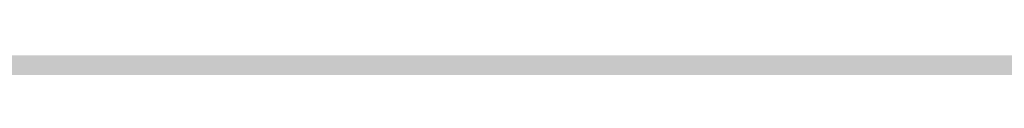
# Model space of a CAD drawing. Units: millimetres. Extents: x 0 to 2267, y 0 to 1823.
# Tile 180 of 256: x 1838.83 to 1841.442, y 1127.384 to 1127.404. Entities that reach past the tile are written whole.
import ezdxf

# ---------------------------------------------------------------- set-up
doc = ezdxf.new("R2010")
doc.units = ezdxf.units.MM
doc.header["$MEASUREMENT"] = 0
doc.layers.add('M-DIMS', color=2, linetype='Continuous', lineweight=25)
doc.layers.add('M-HATC', color=252, linetype='Continuous', lineweight=18)
doc.styles.get("Standard").update_dxf_attribs({"font": 'arial.ttf'})
doc.dimstyles.get("Standard").update_dxf_attribs({"dimtxt": 7, "dimasz": 4, "dimexe": 0.18, "dimexo": 0.0625, "dimgap": 0.09, "dimtad": 0, "dimdec": 0, "dimzin": 0, "dimdsep": 46, "dimtxsty": 'Standard', "dimcen": 0.09, "dimadec": 0, "dimazin": 0, "dimtfac": 1, "dimtdec": 0, "dimtofl": 0, "dimtmove": 0, "dimatfit": 3, "dimfxl": 1, "dimtolj": 1, "dimtzin": 0, "dimarcsym": 0})

# ---------------------------------------------------------------- blocks, each defined once
blk = doc.blocks.new('*D1')
at = {"layer": 'Defpoints', "color": 0, "transparency": 16777216}
for p in [(1593.4289, 1127.4171), (1843.4289, 1127.4171), (1843.4289, 955.6278)]:
    blk.add_point(p, dxfattribs=at)
at = {"layer": 'M-DIMS', "color": 0, "lineweight": -2, "transparency": 16777216}
for p, q in [((1593.4289, 1127.3546), (1593.4289, 955.4478)), ((1843.4289, 1127.3546), (1843.4289, 955.4478)), ((1597.4289, 955.6278), (1710.5582, 955.6278)), ((1839.4289, 955.6278), (1726.2996, 955.6278))]:
    blk.add_line(p, q, dxfattribs=at)
at = {"layer": 'M-DIMS', "color": 0, "transparency": 16777216}
for points in [[(1597.4289, 956.2944), (1597.4289, 954.9611), (1593.4289, 955.6278)], [(1839.4289, 956.2944), (1839.4289, 954.9611), (1843.4289, 955.6278)]]:
    blk.add_solid(points, dxfattribs=at)
at = {"layer": 'M-DIMS', "color": 0, "transparency": 16777216, "insert": (1718.4289, 955.6278), "char_height": 7, "attachment_point": 5}
blk.add_mtext('\\A1;250', dxfattribs=at)

msp = doc.modelspace()

# ---------------------------------------------------------------- hatches: boundary and pattern name
at = {"layer": 'M-HATC'}
h = msp.add_hatch(color=256, dxfattribs=at)
h.dxf.hatch_style = 1
h.paths.add_polyline_path([(2055.771, 1603.062), (1381.0868, 1603.062), (1381.0868, 1598.062), (2055.771, 1598.062)])
h.paths.add_polyline_path([(2055.771, 1598.062), (1381.0868, 1598.062), (1381.0868, 1593.062), (2055.771, 1593.062)])
h.paths.add_polyline_path([(2051.3074, 1536.7609), (1385.5504, 1536.7609), (1385.5504, 1526.7609), (1387.5504, 1526.7609), (1388.5366, 1525.0528), (1385.3319, 1521.2335), (1385.3319, 1521.2226), (2050.2542, 1522.7491), (2048.3212, 1525.0528), (2049.3074, 1526.7609), (2051.3074, 1526.7609)])
edge = h.paths.add_edge_path()
edge.add_arc((1847.5345, 1379.1492), 135, 222.603061, 222.890851, ccw=False)
edge.add_line((1748.1663, 1287.7656), (1683.0921, 1287.7656))
edge.add_arc((1583.7239, 1379.1492), 135, 317.109149, 317.396939, ccw=False)
edge.add_arc((1678.9686, 1290.6707), 5, 222.8909, 317.1091, ccw=False)
edge.add_arc((1774.2133, 1379.1492), 135, 222.603061, 222.890851, ccw=False)
edge.add_line((1674.8451, 1287.7656), (1609.7709, 1287.7656))
edge.add_arc((1510.4027, 1379.1492), 135, 317.109149, 317.396939, ccw=False)
edge.add_arc((1605.6474, 1290.6707), 5, 222.8909, 317.1091, ccw=False)
edge.add_arc((1700.8921, 1379.1492), 135, 222.603061, 222.890851, ccw=False)
edge.add_line((1601.5239, 1287.7656), (1536.4497, 1287.7656))
edge.add_arc((1437.0815, 1379.1492), 135, 317.109149, 317.396939, ccw=False)
edge.add_arc((1532.3262, 1290.6707), 5, 222.8909, 317.1091, ccw=False)
edge.add_arc((1627.5709, 1379.1492), 135, 222.603061, 222.890851, ccw=False)
edge.add_line((1528.2027, 1287.7656), (1505.9289, 1287.7656))
edge.add_spline(control_points=[(1505.9289, 1287.7656), (1504.2622, 1287.7656), (1504.2622, 1282.7656), (1505.9289, 1282.7656)], knot_values=[0, 0, 0, 0, 5, 5, 5, 5], degree=3, periodic=0)
edge.add_line((1505.9289, 1282.7656), (1930.9289, 1282.7656))
edge.add_spline(control_points=[(1930.9289, 1282.7656), (1932.5956, 1282.7656), (1932.5956, 1287.7656), (1930.9289, 1287.7656)], knot_values=[0, 0, 0, 0, 5, 5, 5, 5], degree=3, periodic=0)
edge.add_line((1930.9289, 1287.7656), (1903.0557, 1287.7656))
edge.add_arc((1803.6875, 1379.1492), 135, 317.109149, 317.396939, ccw=False)
edge.add_arc((1898.9322, 1290.6707), 5, 222.8909, 317.1091, ccw=False)
edge.add_arc((1994.1769, 1379.1492), 135, 222.603061, 222.890851, ccw=False)
edge.add_line((1894.8087, 1287.7656), (1829.7345, 1287.7656))
edge.add_arc((1730.3663, 1379.1492), 135, 317.109149, 317.396939, ccw=False)
edge.add_arc((1825.611, 1290.6707), 5, 222.8909, 317.1091, ccw=False)
edge.add_arc((1920.8557, 1379.1492), 135, 222.603061, 222.890851, ccw=False)
edge.add_line((1821.4875, 1287.7656), (1756.4133, 1287.7656))
edge.add_arc((1657.0451, 1379.1492), 135, 317.109149, 317.396939, ccw=False)
edge.add_arc((1752.2898, 1290.6707), 5, 222.8909, 317.1091, ccw=False)
edge = h.paths.add_edge_path()
edge.add_spline(control_points=[(1843.4289, 1227.2475), (1845.0956, 1227.2475), (1845.0956, 1232.2475), (1843.4289, 1232.2475)], knot_values=[0, 0, 0, 0, 5, 5, 5, 5], degree=3, periodic=0)
edge.add_line((1843.4289, 1232.2475), (1593.4289, 1232.2475))
edge.add_spline(control_points=[(1593.4289, 1232.2475), (1591.7622, 1232.2475), (1591.7622, 1227.2475), (1593.4289, 1227.2475)], knot_values=[0, 0, 0, 0, 5, 5, 5, 5], degree=3, periodic=0)
edge.add_line((1593.4289, 1227.2475), (1843.4289, 1227.2475))
h.paths.add_polyline_path([(1905.9289, 1127.4171), (1530.9289, 1127.4171, 0.414214), (1520.9289, 1117.4171), (1530.9289, 1117.4171), (1915.9289, 1117.4171, 0.414214)])
edge = h.paths.add_edge_path()
edge.add_arc((1397.0858, 1498.4078), 12.7299, 90.78215, 190.87871, ccw=False)
edge.add_line((1396.912, 1511.1365), (1428.0097, 1511.3488))
edge.add_line((1428.0097, 1511.3488), (1433.0097, 1511.3488))
edge.add_line((1433.0097, 1511.3488), (1434.439, 1511.3488))
edge.add_arc((1419.474, 1498.0804), 20, 41.561, 74.08211)
edge.add_line((1424.9592, 1517.3135), (1399.9351, 1517.2561))
edge.add_spline(control_points=[(1399.9307, 1517.2561), (1399.884, 1517.2131), (1399.8328, 1517.1689), (1399.7774, 1517.1236)], knot_values=[11.567499, 11.567499, 11.567499, 11.567499, 11.814249, 11.814249, 11.814249, 11.814249], degree=3, periodic=0)
edge.add_spline(control_points=[(1399.6328, 1517.0099), (1399.5831, 1516.9721), (1399.5307, 1516.9338), (1399.4759, 1516.8947)], knot_values=[11.167718, 11.167718, 11.167718, 11.167718, 11.365188, 11.365188, 11.365188, 11.365188], degree=3, periodic=0)
edge.add_spline(control_points=[(1399.3398, 1516.8001), (1399.1514, 1516.6719), (1398.9384, 1516.5377), (1398.704, 1516.3994)], knot_values=[10.376405, 10.376405, 10.376405, 10.376405, 11.00994, 11.00994, 11.00994, 11.00994], degree=3, periodic=0)
edge.add_spline(control_points=[(1398.6572, 1516.3719), (1398.5789, 1516.326), (1398.4983, 1516.2797), (1398.4155, 1516.2331)], knot_values=[10.125175, 10.125175, 10.125175, 10.125175, 10.334406, 10.334406, 10.334406, 10.334406], degree=3, periodic=0)
edge.add_spline(control_points=[(1398.2642, 1516.1487), (1398.196, 1516.1111), (1398.1263, 1516.0732), (1398.0555, 1516.0351)], knot_values=[9.832246, 9.832246, 9.832246, 9.832246, 9.999658, 9.999658, 9.999658, 9.999658], degree=3, periodic=0)
edge.add_spline(control_points=[(1397.9987, 1516.0048), (1397.7312, 1515.8621), (1397.446, 1515.7171), (1397.1466, 1515.5714)], knot_values=[9.161808, 9.161808, 9.161808, 9.161808, 9.787769, 9.787769, 9.787769, 9.787769], degree=3, periodic=0)
edge.add_spline(control_points=[(1397.1466, 1515.5714), (1396.8418, 1515.423), (1396.5222, 1515.274), (1396.1914, 1515.1262)], knot_values=[8.524455, 8.524455, 8.524455, 8.524455, 9.161808, 9.161808, 9.161808, 9.161808], degree=3, periodic=0)
edge.add_spline(control_points=[(1396.0777, 1515.0756), (1395.9854, 1515.0348), (1395.8922, 1514.994), (1395.7983, 1514.9534)], knot_values=[8.275193, 8.275193, 8.275193, 8.275193, 8.451726, 8.451726, 8.451726, 8.451726], degree=3, periodic=0)
edge.add_spline(control_points=[(1395.6018, 1514.8691), (1395.4997, 1514.8257), (1395.3968, 1514.7824), (1395.2932, 1514.7394)], knot_values=[7.962917, 7.962917, 7.962917, 7.962917, 8.152764, 8.152764, 8.152764, 8.152764], degree=3, periodic=0)
edge.add_spline(control_points=[(1395.2116, 1514.7057), (1394.8278, 1514.5475), (1394.4345, 1514.3929), (1394.0364, 1514.2442)], knot_values=[7.21254, 7.21254, 7.21254, 7.21254, 7.913148, 7.913148, 7.913148, 7.913148], degree=3, periodic=0)
edge.add_spline(control_points=[(1394.0364, 1514.2442), (1393.7076, 1514.1214), (1393.3754, 1514.0027), (1393.0427, 1513.8895)], knot_values=[6.633733, 6.633733, 6.633733, 6.633733, 7.21254, 7.21254, 7.21254, 7.21254], degree=3, periodic=0)
edge.add_spline(control_points=[(1392.8214, 1513.815), (1392.7198, 1513.7812), (1392.6181, 1513.7479), (1392.5166, 1513.7152)], knot_values=[6.328796, 6.328796, 6.328796, 6.328796, 6.505493, 6.505493, 6.505493, 6.505493], degree=3, periodic=0)
edge.add_spline(control_points=[(1392.5166, 1513.7152), (1392.3187, 1513.6515), (1392.1212, 1513.59), (1391.9244, 1513.531)], knot_values=[5.984605, 5.984605, 5.984605, 5.984605, 6.328796, 6.328796, 6.328796, 6.328796], degree=3, periodic=0)
edge.add_spline(control_points=[(1391.7915, 1513.4915), (1391.3122, 1513.3501), (1390.8384, 1513.2239), (1390.3784, 1513.1171)], knot_values=[5.066697, 5.066697, 5.066697, 5.066697, 5.907055, 5.907055, 5.907055, 5.907055], degree=3, periodic=0)
edge.add_spline(control_points=[(1390.3784, 1513.1171), (1390.1797, 1513.071), (1389.9836, 1513.0284), (1389.7907, 1512.9899)], knot_values=[4.70367, 4.70367, 4.70367, 4.70367, 5.066695, 5.066695, 5.066695, 5.066695], degree=3, periodic=0)
edge.add_spline(control_points=[(1389.422, 1512.9204), (1389.2459, 1512.8892), (1389.0729, 1512.8617), (1388.9036, 1512.8381)], knot_values=[4.130571, 4.130571, 4.130571, 4.130571, 4.469816, 4.469816, 4.469816, 4.469816], degree=3, periodic=0)
edge.add_spline(control_points=[(1388.9036, 1512.8381), (1388.591, 1512.7946), (1388.2911, 1512.7644), (1388.0071, 1512.7494)], knot_values=[3.504031, 3.504031, 3.504031, 3.504031, 4.130571, 4.130571, 4.130571, 4.130571], degree=3, periodic=0)
edge.add_spline(control_points=[(1387.9356, 1512.7459), (1387.8538, 1512.7423), (1387.7733, 1512.74), (1387.6944, 1512.739)], knot_values=[3.268866, 3.268866, 3.268866, 3.268866, 3.451164, 3.451164, 3.451164, 3.451164], degree=3, periodic=0)
edge.add_spline(control_points=[(1387.3351, 1512.7443), (1387.2076, 1512.7499), (1387.0847, 1512.7597), (1386.967, 1512.7739)], knot_values=[2.670686, 2.670686, 2.670686, 2.670686, 2.984, 2.984, 2.984, 2.984], degree=3, periodic=0)
edge.add_spline(control_points=[(1386.8327, 1512.7922), (1386.8209, 1512.7941), (1386.8092, 1512.7959), (1386.7975, 1512.7979)], knot_values=[2.516981, 2.516981, 2.516981, 2.516981, 2.549528, 2.549528, 2.549528, 2.549528], degree=3, periodic=0)
edge.add_spline(control_points=[(1386.4526, 1512.8735), (1386.4257, 1512.881), (1386.3993, 1512.889), (1386.3733, 1512.8972)], knot_values=[2.095869, 2.095869, 2.095869, 2.095869, 2.17941, 2.17941, 2.17941, 2.17941], degree=3, periodic=0)
edge.add_spline(control_points=[(1386.0691, 1513.0189), (1386.0634, 1513.0217), (1386.0577, 1513.0246), (1386.052, 1513.0275)], knot_values=[1.72453, 1.72453, 1.72453, 1.72453, 1.745933, 1.745933, 1.745933, 1.745933], degree=3, periodic=0)
edge.add_arc((1399.474, 1498.0804), 20, 131.82432, 180)
edge.add_arc((1630.3336, 1505.5484), 250.9708, 181.705176, 236.427975)
edge.add_arc((1605.3399, 1483.3044), 218.7822, 238.660829, 243.34961)
edge.add_arc((1647.0911, 1510.3592), 262.8986, 183.129836, 237.853442, ccw=False)
h.paths.add_polyline_path([(1406.5369, 1391.9644, 0.149382), (1491.5506, 1296.4418, -0.129517)], flags=17)
edge = h.paths.add_edge_path()
edge.add_arc((2037.3838, 1498.0804), 20, 0, 48.26587)
edge.add_spline(control_points=[(2050.6973, 1513.0052), (2050.6512, 1512.9847), (2050.6034, 1512.9655), (2050.5539, 1512.9477)], knot_values=[1.835652, 1.835652, 1.835652, 1.835652, 2.000781, 2.000781, 2.000781, 2.000781], degree=3, periodic=0)
edge.add_spline(control_points=[(2050.4616, 1512.9166), (2050.479, 1512.9221), (2050.4963, 1512.9277), (2050.5133, 1512.9335)], knot_values=[2.045477, 2.045477, 2.045477, 2.045477, 2.101389, 2.101389, 2.101389, 2.101389], degree=3, periodic=0)
edge.add_spline(control_points=[(2050.129, 1512.8342), (2050.1984, 1512.8473), (2050.2657, 1512.8623), (2050.3308, 1512.8792)], knot_values=[2.237629, 2.237629, 2.237629, 2.237629, 2.435841, 2.435841, 2.435841, 2.435841], degree=3, periodic=0)
edge.add_spline(control_points=[(2050.0946, 1512.8278), (2050.1061, 1512.8299), (2050.1176, 1512.832), (2050.129, 1512.8342)], knot_values=[2.435841, 2.435841, 2.435841, 2.435841, 2.468321, 2.468321, 2.468321, 2.468321], degree=3, periodic=0)
edge.add_spline(control_points=[(2049.7843, 1512.7851), (2049.8552, 1512.7922), (2049.9243, 1512.8008), (2049.9917, 1512.8109)], knot_values=[2.563852, 2.563852, 2.563852, 2.563852, 2.748541, 2.748541, 2.748541, 2.748541], degree=3, periodic=0)
edge.add_spline(control_points=[(2049.4052, 1512.7617), (2049.5364, 1512.7653), (2049.6629, 1512.773), (2049.7843, 1512.7851)], knot_values=[2.748541, 2.748541, 2.748541, 2.748541, 3.064882, 3.064882, 3.064882, 3.064882], degree=3, periodic=0)
edge.add_spline(control_points=[(2049.1698, 1512.7597), (2049.2336, 1512.7591), (2049.2965, 1512.7594), (2049.3584, 1512.7606)], knot_values=[3.102309, 3.102309, 3.102309, 3.102309, 3.2503, 3.2503, 3.2503, 3.2503], degree=3, periodic=0)
edge.add_spline(control_points=[(2048.8573, 1512.7691), (2048.9638, 1512.7638), (2049.068, 1512.7606), (2049.1698, 1512.7597)], knot_values=[3.2503, 3.2503, 3.2503, 3.2503, 3.486069, 3.486069, 3.486069, 3.486069], degree=3, periodic=0)
edge.add_spline(control_points=[(2048.6924, 1512.7789), (2048.3729, 1512.8009), (2048.0345, 1512.8411), (2047.6817, 1512.897)], knot_values=[3.606429, 3.606429, 3.606429, 3.606429, 4.2989, 4.2989, 4.2989, 4.2989], degree=3, periodic=0)
edge.add_spline(control_points=[(2047.6817, 1512.897), (2047.5458, 1512.9185), (2047.4077, 1512.9424), (2047.2678, 1512.9685)], knot_values=[4.2989, 4.2989, 4.2989, 4.2989, 4.565769, 4.565769, 4.565769, 4.565769], degree=3, periodic=0)
edge.add_spline(control_points=[(2047.2678, 1512.9685), (2047.1449, 1512.9914), (2047.0207, 1513.016), (2046.8951, 1513.0422)], knot_values=[4.565769, 4.565769, 4.565769, 4.565769, 4.799971, 4.799971, 4.799971, 4.799971], degree=3, periodic=0)
edge.add_spline(control_points=[(2046.8951, 1513.0422), (2046.5286, 1513.1188), (2046.1513, 1513.209), (2045.7676, 1513.3107)], knot_values=[4.799971, 4.799971, 4.799971, 4.799971, 5.483718, 5.483718, 5.483718, 5.483718], degree=3, periodic=0)
edge.add_spline(control_points=[(2045.7676, 1513.3107), (2045.3724, 1513.4154), (2044.9704, 1513.5322), (2044.5662, 1513.6588)], knot_values=[5.483718, 5.483718, 5.483718, 5.483718, 6.187866, 6.187866, 6.187866, 6.187866], degree=3, periodic=0)
edge.add_spline(control_points=[(2044.5662, 1513.6588), (2044.4149, 1513.7061), (2044.2633, 1513.7549), (2044.1116, 1513.8048)], knot_values=[6.187866, 6.187866, 6.187866, 6.187866, 6.451551, 6.451551, 6.451551, 6.451551], degree=3, periodic=0)
edge.add_spline(control_points=[(2044.1116, 1513.8048), (2043.9967, 1513.8427), (2043.8817, 1513.8813), (2043.7668, 1513.9205)], knot_values=[6.451551, 6.451551, 6.451551, 6.451551, 6.651434, 6.651434, 6.651434, 6.651434], degree=3, periodic=0)
edge.add_spline(control_points=[(2043.7668, 1513.9205), (2043.3716, 1514.0554), (2042.9774, 1514.1979), (2042.5886, 1514.3458)], knot_values=[6.651434, 6.651434, 6.651434, 6.651434, 7.338879, 7.338879, 7.338879, 7.338879], degree=3, periodic=0)
edge.add_spline(control_points=[(2042.5886, 1514.3458), (2042.1643, 1514.5071), (2041.7465, 1514.6749), (2041.3409, 1514.846)], knot_values=[7.338879, 7.338879, 7.338879, 7.338879, 8.089209, 8.089209, 8.089209, 8.089209], degree=3, periodic=0)
edge.add_spline(control_points=[(2041.3409, 1514.846), (2041.1028, 1514.9465), (2040.869, 1515.0481), (2040.6405, 1515.1502)], knot_values=[8.089209, 8.089209, 8.089209, 8.089209, 8.529587, 8.529587, 8.529587, 8.529587], degree=3, periodic=0)
edge.add_spline(control_points=[(2040.51, 1515.2089), (2040.0824, 1515.4022), (2039.6747, 1515.5971), (2039.295, 1515.7894)], knot_values=[8.613818, 8.613818, 8.613818, 8.613818, 9.44571, 9.44571, 9.44571, 9.44571], degree=3, periodic=0)
edge.add_spline(control_points=[(2039.295, 1515.7894), (2039.0618, 1515.9075), (2038.8391, 1516.0246), (2038.6288, 1516.1398)], knot_values=[9.44571, 9.44571, 9.44571, 9.44571, 9.956404, 9.956404, 9.956404, 9.956404], degree=3, periodic=0)
edge.add_spline(control_points=[(2038.6288, 1516.1398), (2038.5187, 1516.2001), (2038.4121, 1516.2598), (2038.309, 1516.3189)], knot_values=[9.956404, 9.956404, 9.956404, 9.956404, 10.223542, 10.223542, 10.223542, 10.223542], degree=3, periodic=0)
edge.add_spline(control_points=[(2038.309, 1516.3189), (2038.2138, 1516.3735), (2038.1216, 1516.4276), (2038.0328, 1516.481)], knot_values=[10.223542, 10.223542, 10.223542, 10.223542, 10.47051, 10.47051, 10.47051, 10.47051], degree=3, periodic=0)
edge.add_spline(control_points=[(2038.0328, 1516.481), (2037.7855, 1516.6296), (2037.5639, 1516.773), (2037.3722, 1516.909)], knot_values=[10.47051, 10.47051, 10.47051, 10.47051, 11.15767, 11.15767, 11.15767, 11.15767], degree=3, periodic=0)
edge.add_spline(control_points=[(2037.3722, 1516.909), (2037.2789, 1516.9752), (2037.1927, 1517.0396), (2037.1142, 1517.102)], knot_values=[11.15767, 11.15767, 11.15767, 11.15767, 11.49227, 11.49227, 11.49227, 11.49227], degree=3, periodic=0)
edge.add_spline(control_points=[(2036.8564, 1517.3259), (2036.9148, 1517.2692), (2036.9814, 1517.2103), (2037.0557, 1517.1492)], knot_values=[11.577341, 11.577341, 11.577341, 11.577341, 11.91035, 11.91035, 11.91035, 11.91035], degree=3, periodic=0)
edge.add_spline(control_points=[(2036.8074, 1517.3748), (2036.823, 1517.3587), (2036.8393, 1517.3424), (2036.8564, 1517.3259)], knot_values=[11.91035, 11.91035, 11.91035, 11.91035, 12.007402, 12.007402, 12.007402, 12.007402], degree=3, periodic=0)
edge.add_spline(control_points=[(2036.7017, 1517.494), (2036.7104, 1517.483), (2036.7196, 1517.4719), (2036.7291, 1517.4606)], knot_values=[12.184155, 12.184155, 12.184155, 12.184155, 12.255409, 12.255409, 12.255409, 12.255409], degree=3, periodic=0)
edge.add_spline(control_points=[(2036.6159, 1517.6205), (2036.62, 1517.613), (2036.6243, 1517.6055), (2036.6289, 1517.5979)], knot_values=[12.487913, 12.487913, 12.487913, 12.487913, 12.541035, 12.541035, 12.541035, 12.541035], degree=3, periodic=0)
edge.add_spline(control_points=[(2036.5635, 1517.786), (2036.5637, 1517.7794), (2036.5642, 1517.7726), (2036.565, 1517.7658)], knot_values=[12.911761, 12.911761, 12.911761, 12.911761, 12.968286, 12.968286, 12.968286, 12.968286], degree=3, periodic=0)
edge.add_spline(control_points=[(2036.6166, 1517.9304), (2036.6125, 1517.9259), (2036.6086, 1517.9212), (2036.6049, 1517.9165)], knot_values=[13.382527, 13.382527, 13.382527, 13.382527, 13.433791, 13.433791, 13.433791, 13.433791], degree=3, periodic=0)
edge.add_spline(control_points=[(2036.749, 1518.017), (2036.7361, 1518.0116), (2036.7239, 1518.006), (2036.7124, 1518.0002)], knot_values=[13.726299, 13.726299, 13.726299, 13.726299, 13.809928, 13.809928, 13.809928, 13.809928], degree=3, periodic=0)
edge.add_spline(control_points=[(2036.8604, 1518.0528), (2036.8386, 1518.0474), (2036.8181, 1518.0416), (2036.7988, 1518.0353)], knot_values=[13.910887, 13.910887, 13.910887, 13.910887, 14.02153, 14.02153, 14.02153, 14.02153], degree=3, periodic=0)
edge.add_line((2036.9639, 1518.0804), (2032.3838, 1518.0804))
edge.add_line((2032.3838, 1518.0804), (2027.3838, 1518.0804))
edge.add_line((2027.3838, 1518.0804), (2022.3838, 1518.0804))
edge.add_line((2022.3838, 1518.0804), (2017.3838, 1518.0804))
edge.add_arc((2017.3838, 1498.0804), 20, 90, 138.439)
edge.add_line((2002.4188, 1511.3488), (2003.8481, 1511.3488))
edge.add_line((2003.8481, 1511.3488), (2008.8481, 1511.3488))
edge.add_line((2008.8481, 1511.3488), (2039.772, 1511.1377))
edge.add_arc((2039.772, 1498.4078), 12.7299, -10.87871, 90, ccw=False)
edge.add_arc((1789.7668, 1510.3592), 262.8986, 302.146558, 356.870164, ccw=False)
edge.add_arc((1831.5179, 1483.3044), 218.7822, 296.65039, 301.339171)
edge.add_arc((1806.5242, 1505.5484), 250.9708, 303.572025, 358.294824)
h.paths.add_polyline_path([(2030.321, 1391.9644, -0.129517), (1945.3072, 1296.4418, 0.149382)], flags=17)
edge = h.paths.add_edge_path()
edge.add_spline(control_points=[(2037.2464, 1518.0821), (2037.2898, 1518.081), (2037.3355, 1518.0804), (2037.3838, 1518.0804)], knot_values=[0.000012, 0.000012, 0.000012, 0.000012, 0.144754, 0.144754, 0.144754, 0.144754], degree=3, periodic=0)
edge.add_line((2037.3357, 1518.0804), (2037.0096, 1518.0804))
edge.add_spline(control_points=[(2037.0096, 1518.0804), (2036.9822, 1518.0768), (2036.956, 1518.0727), (2036.9312, 1518.0681)], knot_values=[14.13465, 14.13465, 14.13465, 14.13465, 14.247197, 14.247197, 14.247197, 14.247197], degree=3, periodic=0)
edge.add_spline(control_points=[(2036.9312, 1518.0681), (2036.9276, 1518.0674), (2036.9241, 1518.0667), (2036.9205, 1518.0661)], knot_values=[14.118315, 14.118315, 14.118315, 14.118315, 14.13465, 14.13465, 14.13465, 14.13465], degree=3, periodic=0)
edge.add_spline(control_points=[(2036.9205, 1518.0661), (2036.9118, 1518.0644), (2036.9032, 1518.0626), (2036.8948, 1518.0608)], knot_values=[14.078086, 14.078086, 14.078086, 14.078086, 14.118315, 14.118315, 14.118315, 14.118315], degree=3, periodic=0)
edge.add_spline(control_points=[(2036.8948, 1518.0608), (2036.883, 1518.0583), (2036.8716, 1518.0556), (2036.8604, 1518.0528)], knot_values=[14.02153, 14.02153, 14.02153, 14.02153, 14.078086, 14.078086, 14.078086, 14.078086], degree=3, periodic=0)
edge.add_spline(control_points=[(2036.8604, 1518.0528), (2036.8386, 1518.0474), (2036.8181, 1518.0416), (2036.7988, 1518.0353)], knot_values=[13.910887, 13.910887, 13.910887, 13.910887, 14.02153, 14.02153, 14.02153, 14.02153], degree=3, periodic=0)
edge.add_spline(control_points=[(2036.7988, 1518.0353), (2036.7981, 1518.035), (2036.7974, 1518.0348), (2036.7967, 1518.0346)], knot_values=[13.906906, 13.906906, 13.906906, 13.906906, 13.910887, 13.910887, 13.910887, 13.910887], degree=3, periodic=0)
edge.add_spline(control_points=[(2036.7967, 1518.0346), (2036.7882, 1518.0318), (2036.7799, 1518.0289), (2036.7719, 1518.0259)], knot_values=[13.857826, 13.857826, 13.857826, 13.857826, 13.906906, 13.906906, 13.906906, 13.906906], degree=3, periodic=0)
edge.add_spline(control_points=[(2036.7719, 1518.0259), (2036.764, 1518.023), (2036.7564, 1518.02), (2036.749, 1518.017)], knot_values=[13.809928, 13.809928, 13.809928, 13.809928, 13.857826, 13.857826, 13.857826, 13.857826], degree=3, periodic=0)
edge.add_spline(control_points=[(2036.749, 1518.017), (2036.7361, 1518.0116), (2036.7239, 1518.006), (2036.7124, 1518.0002)], knot_values=[13.726299, 13.726299, 13.726299, 13.726299, 13.809928, 13.809928, 13.809928, 13.809928], degree=3, periodic=0)
edge.add_spline(control_points=[(2036.7124, 1518.0002), (2036.7121, 1518), (2036.7118, 1517.9999), (2036.7115, 1517.9997)], knot_values=[13.723993, 13.723993, 13.723993, 13.723993, 13.726299, 13.726299, 13.726299, 13.726299], degree=3, periodic=0)
edge.add_spline(control_points=[(2036.7115, 1517.9997), (2036.7063, 1517.9971), (2036.7013, 1517.9944), (2036.6965, 1517.9917)], knot_values=[13.686536, 13.686536, 13.686536, 13.686536, 13.723993, 13.723993, 13.723993, 13.723993], degree=3, periodic=0)
edge.add_spline(control_points=[(2036.6965, 1517.9917), (2036.6919, 1517.9891), (2036.6874, 1517.9865), (2036.6831, 1517.9839)], knot_values=[13.651251, 13.651251, 13.651251, 13.651251, 13.686536, 13.686536, 13.686536, 13.686536], degree=3, periodic=0)
edge.add_spline(control_points=[(2036.6831, 1517.9839), (2036.6764, 1517.9798), (2036.67, 1517.9757), (2036.6639, 1517.9714)], knot_values=[13.596804, 13.596804, 13.596804, 13.596804, 13.651251, 13.651251, 13.651251, 13.651251], degree=3, periodic=0)
edge.add_spline(control_points=[(2036.6639, 1517.9714), (2036.6636, 1517.9712), (2036.6633, 1517.9709), (2036.6629, 1517.9707)], knot_values=[13.593956, 13.593956, 13.593956, 13.593956, 13.596804, 13.596804, 13.596804, 13.596804], degree=3, periodic=0)
edge.add_spline(control_points=[(2036.6629, 1517.9707), (2036.6603, 1517.9689), (2036.6577, 1517.967), (2036.6552, 1517.9651)], knot_values=[13.570322, 13.570322, 13.570322, 13.570322, 13.593956, 13.593956, 13.593956, 13.593956], degree=3, periodic=0)
edge.add_spline(control_points=[(2036.6552, 1517.9651), (2036.6525, 1517.9631), (2036.6499, 1517.9611), (2036.6474, 1517.9591)], knot_values=[13.545477, 13.545477, 13.545477, 13.545477, 13.570322, 13.570322, 13.570322, 13.570322], degree=3, periodic=0)
edge.add_spline(control_points=[(2036.6474, 1517.9591), (2036.6472, 1517.9589), (2036.6471, 1517.9588), (2036.6469, 1517.9587)], knot_values=[13.543931, 13.543931, 13.543931, 13.543931, 13.545477, 13.545477, 13.545477, 13.545477], degree=3, periodic=0)
edge.add_spline(control_points=[(2036.6469, 1517.9587), (2036.6412, 1517.9541), (2036.6358, 1517.9494), (2036.6307, 1517.9447)], knot_values=[13.488237, 13.488237, 13.488237, 13.488237, 13.543931, 13.543931, 13.543931, 13.543931], degree=3, periodic=0)
edge.add_spline(control_points=[(2036.6307, 1517.9447), (2036.6282, 1517.9423), (2036.6257, 1517.9399), (2036.6233, 1517.9374)], knot_values=[13.460307, 13.460307, 13.460307, 13.460307, 13.488237, 13.488237, 13.488237, 13.488237], degree=3, periodic=0)
edge.add_spline(control_points=[(2036.6233, 1517.9374), (2036.6215, 1517.9356), (2036.6198, 1517.9338), (2036.6181, 1517.932)], knot_values=[13.439712, 13.439712, 13.439712, 13.439712, 13.460307, 13.460307, 13.460307, 13.460307], degree=3, periodic=0)
edge.add_spline(control_points=[(2036.6181, 1517.932), (2036.6176, 1517.9315), (2036.6171, 1517.9309), (2036.6166, 1517.9304)], knot_values=[13.433791, 13.433791, 13.433791, 13.433791, 13.439712, 13.439712, 13.439712, 13.439712], degree=3, periodic=0)
edge.add_spline(control_points=[(2036.6166, 1517.9304), (2036.6125, 1517.9259), (2036.6086, 1517.9212), (2036.6049, 1517.9165)], knot_values=[13.382527, 13.382527, 13.382527, 13.382527, 13.433791, 13.433791, 13.433791, 13.433791], degree=3, periodic=0)
edge.add_spline(control_points=[(2036.6049, 1517.9165), (2036.6026, 1517.9135), (2036.6004, 1517.9104), (2036.5982, 1517.9074)], knot_values=[13.350017, 13.350017, 13.350017, 13.350017, 13.382527, 13.382527, 13.382527, 13.382527], degree=3, periodic=0)
edge.add_spline(control_points=[(2036.5982, 1517.9074), (2036.5972, 1517.9059), (2036.5962, 1517.9043), (2036.5952, 1517.9028)], knot_values=[13.333922, 13.333922, 13.333922, 13.333922, 13.350017, 13.350017, 13.350017, 13.350017], degree=3, periodic=0)
edge.add_spline(control_points=[(2036.5952, 1517.9028), (2036.5945, 1517.9018), (2036.5939, 1517.9009), (2036.5933, 1517.8999)], knot_values=[13.323828, 13.323828, 13.323828, 13.323828, 13.333922, 13.333922, 13.333922, 13.333922], degree=3, periodic=0)
edge.add_spline(control_points=[(2036.5933, 1517.8999), (2036.5905, 1517.8955), (2036.5879, 1517.8909), (2036.5855, 1517.8864)], knot_values=[13.277545, 13.277545, 13.277545, 13.277545, 13.323828, 13.323828, 13.323828, 13.323828], degree=3, periodic=0)
edge.add_spline(control_points=[(2036.5855, 1517.8864), (2036.5836, 1517.8827), (2036.5817, 1517.8789), (2036.5801, 1517.8751)], knot_values=[13.240119, 13.240119, 13.240119, 13.240119, 13.277545, 13.277545, 13.277545, 13.277545], degree=3, periodic=0)
edge.add_spline(control_points=[(2036.5801, 1517.8751), (2036.5795, 1517.8739), (2036.579, 1517.8727), (2036.5785, 1517.8715)], knot_values=[13.228211, 13.228211, 13.228211, 13.228211, 13.240119, 13.240119, 13.240119, 13.240119], degree=3, periodic=0)
edge.add_spline(control_points=[(2036.5785, 1517.8715), (2036.578, 1517.8702), (2036.5774, 1517.869), (2036.5769, 1517.8677)], knot_values=[13.215717, 13.215717, 13.215717, 13.215717, 13.228211, 13.228211, 13.228211, 13.228211], degree=3, periodic=0)
edge.add_spline(control_points=[(2036.5769, 1517.8677), (2036.5755, 1517.864), (2036.5741, 1517.8603), (2036.5729, 1517.8565)], knot_values=[13.179847, 13.179847, 13.179847, 13.179847, 13.215717, 13.215717, 13.215717, 13.215717], degree=3, periodic=0)
edge.add_spline(control_points=[(2036.5729, 1517.8565), (2036.5713, 1517.8515), (2036.5699, 1517.8464), (2036.5687, 1517.8413)], knot_values=[13.132017, 13.132017, 13.132017, 13.132017, 13.179847, 13.179847, 13.179847, 13.179847], degree=3, periodic=0)
edge.add_spline(control_points=[(2036.5687, 1517.8413), (2036.5684, 1517.8402), (2036.5682, 1517.8392), (2036.568, 1517.8382)], knot_values=[13.122482, 13.122482, 13.122482, 13.122482, 13.132017, 13.132017, 13.132017, 13.132017], degree=3, periodic=0)
edge.add_spline(control_points=[(2036.568, 1517.8382), (2036.5676, 1517.8363), (2036.5672, 1517.8345), (2036.5669, 1517.8327)], knot_values=[13.105592, 13.105592, 13.105592, 13.105592, 13.122482, 13.122482, 13.122482, 13.122482], degree=3, periodic=0)
edge.add_spline(control_points=[(2036.5669, 1517.8327), (2036.5662, 1517.8292), (2036.5657, 1517.8257), (2036.5652, 1517.8222)], knot_values=[13.074063, 13.074063, 13.074063, 13.074063, 13.105592, 13.105592, 13.105592, 13.105592], degree=3, periodic=0)
edge.add_spline(control_points=[(2036.5652, 1517.8222), (2036.5652, 1517.8222), (2036.5652, 1517.8222), (2036.5652, 1517.8222)], knot_values=[13.074043, 13.074043, 13.074043, 13.074043, 13.074063, 13.074063, 13.074063, 13.074063], degree=3, periodic=0)
edge.add_spline(control_points=[(2036.5652, 1517.8222), (2036.5644, 1517.8164), (2036.5639, 1517.8106), (2036.5636, 1517.8046)], knot_values=[13.021884, 13.021884, 13.021884, 13.021884, 13.074043, 13.074043, 13.074043, 13.074043], degree=3, periodic=0)
edge.add_spline(control_points=[(2036.5636, 1517.8046), (2036.5636, 1517.804), (2036.5636, 1517.8034), (2036.5635, 1517.8028)], knot_values=[13.01674, 13.01674, 13.01674, 13.01674, 13.021884, 13.021884, 13.021884, 13.021884], degree=3, periodic=0)
edge.add_spline(control_points=[(2036.5635, 1517.8028), (2036.5634, 1517.8005), (2036.5634, 1517.7982), (2036.5634, 1517.7958)], knot_values=[12.996438, 12.996438, 12.996438, 12.996438, 13.01674, 13.01674, 13.01674, 13.01674], degree=3, periodic=0)
edge.add_spline(control_points=[(2036.5634, 1517.7958), (2036.5633, 1517.7926), (2036.5634, 1517.7893), (2036.5635, 1517.786)], knot_values=[12.968286, 12.968286, 12.968286, 12.968286, 12.996438, 12.996438, 12.996438, 12.996438], degree=3, periodic=0)
edge.add_spline(control_points=[(2036.5635, 1517.786), (2036.5637, 1517.7794), (2036.5642, 1517.7726), (2036.565, 1517.7658)], knot_values=[12.911761, 12.911761, 12.911761, 12.911761, 12.968286, 12.968286, 12.968286, 12.968286], degree=3, periodic=0)
edge.add_spline(control_points=[(2036.565, 1517.7658), (2036.565, 1517.7657), (2036.565, 1517.7656), (2036.565, 1517.7656)], knot_values=[12.911017, 12.911017, 12.911017, 12.911017, 12.911761, 12.911761, 12.911761, 12.911761], degree=3, periodic=0)
edge.add_spline(control_points=[(2036.565, 1517.7656), (2036.5654, 1517.7625), (2036.5658, 1517.7593), (2036.5663, 1517.7562)], knot_values=[12.88528, 12.88528, 12.88528, 12.88528, 12.911017, 12.911017, 12.911017, 12.911017], degree=3, periodic=0)
edge.add_spline(control_points=[(2036.5663, 1517.7562), (2036.5667, 1517.7534), (2036.5672, 1517.7506), (2036.5677, 1517.7478)], knot_values=[12.862519, 12.862519, 12.862519, 12.862519, 12.88528, 12.88528, 12.88528, 12.88528], degree=3, periodic=0)
edge.add_spline(control_points=[(2036.5677, 1517.7478), (2036.5678, 1517.7474), (2036.5679, 1517.7469), (2036.568, 1517.7465)], knot_values=[12.858885, 12.858885, 12.858885, 12.858885, 12.862519, 12.862519, 12.862519, 12.862519], degree=3, periodic=0)
edge.add_spline(control_points=[(2036.568, 1517.7465), (2036.5692, 1517.7399), (2036.5707, 1517.7332), (2036.5724, 1517.7264)], knot_values=[12.8053, 12.8053, 12.8053, 12.8053, 12.858885, 12.858885, 12.858885, 12.858885], degree=3, periodic=0)
edge.add_spline(control_points=[(2036.5724, 1517.7264), (2036.5734, 1517.7226), (2036.5745, 1517.7187), (2036.5756, 1517.7149)], knot_values=[12.775176, 12.775176, 12.775176, 12.775176, 12.8053, 12.8053, 12.8053, 12.8053], degree=3, periodic=0)
edge.add_spline(control_points=[(2036.5756, 1517.7149), (2036.5763, 1517.7125), (2036.577, 1517.7102), (2036.5778, 1517.7078)], knot_values=[12.756759, 12.756759, 12.756759, 12.756759, 12.775176, 12.775176, 12.775176, 12.775176], degree=3, periodic=0)
edge.add_spline(control_points=[(2036.5778, 1517.7078), (2036.5781, 1517.7067), (2036.5784, 1517.7057), (2036.5787, 1517.7047)], knot_values=[12.748742, 12.748742, 12.748742, 12.748742, 12.756759, 12.756759, 12.756759, 12.756759], degree=3, periodic=0)
edge.add_spline(control_points=[(2036.5787, 1517.7047), (2036.5808, 1517.6983), (2036.5831, 1517.6919), (2036.5856, 1517.6854)], knot_values=[12.69959, 12.69959, 12.69959, 12.69959, 12.748742, 12.748742, 12.748742, 12.748742], degree=3, periodic=0)
edge.add_spline(control_points=[(2036.5856, 1517.6854), (2036.5876, 1517.68), (2036.5898, 1517.6746), (2036.5921, 1517.6692)], knot_values=[12.659038, 12.659038, 12.659038, 12.659038, 12.69959, 12.69959, 12.69959, 12.69959], degree=3, periodic=0)
edge.add_spline(control_points=[(2036.5921, 1517.6692), (2036.594, 1517.6648), (2036.5959, 1517.6605), (2036.5979, 1517.6561)], knot_values=[12.626806, 12.626806, 12.626806, 12.626806, 12.659038, 12.659038, 12.659038, 12.659038], degree=3, periodic=0)
edge.add_spline(control_points=[(2036.5979, 1517.6561), (2036.5984, 1517.6551), (2036.5989, 1517.6541), (2036.5993, 1517.6531)], knot_values=[12.619394, 12.619394, 12.619394, 12.619394, 12.626806, 12.626806, 12.626806, 12.626806], degree=3, periodic=0)
edge.add_spline(control_points=[(2036.5993, 1517.6531), (2036.6043, 1517.6424), (2036.6099, 1517.6315), (2036.6159, 1517.6205)], knot_values=[12.541039, 12.541039, 12.541039, 12.541039, 12.619394, 12.619394, 12.619394, 12.619394], degree=3, periodic=0)
edge.add_spline(control_points=[(2036.6159, 1517.6205), (2036.6159, 1517.6205), (2036.6159, 1517.6205), (2036.6159, 1517.6205)], knot_values=[12.541035, 12.541035, 12.541035, 12.541035, 12.541039, 12.541039, 12.541039, 12.541039], degree=3, periodic=0)
edge.add_spline(control_points=[(2036.6159, 1517.6205), (2036.62, 1517.613), (2036.6243, 1517.6055), (2036.6289, 1517.5979)], knot_values=[12.487913, 12.487913, 12.487913, 12.487913, 12.541035, 12.541035, 12.541035, 12.541035], degree=3, periodic=0)
edge.add_spline(control_points=[(2036.6289, 1517.5979), (2036.6326, 1517.5916), (2036.6365, 1517.5853), (2036.6406, 1517.5789)], knot_values=[12.443982, 12.443982, 12.443982, 12.443982, 12.487913, 12.487913, 12.487913, 12.487913], degree=3, periodic=0)
edge.add_spline(control_points=[(2036.6406, 1517.5789), (2036.6414, 1517.5776), (2036.6423, 1517.5763), (2036.6431, 1517.5749)], knot_values=[12.434996, 12.434996, 12.434996, 12.434996, 12.443982, 12.443982, 12.443982, 12.443982], degree=3, periodic=0)
edge.add_spline(control_points=[(2036.6431, 1517.5749), (2036.6531, 1517.5596), (2036.6639, 1517.5439), (2036.6756, 1517.528)], knot_values=[12.329647, 12.329647, 12.329647, 12.329647, 12.434996, 12.434996, 12.434996, 12.434996], degree=3, periodic=0)
edge.add_spline(control_points=[(2036.6756, 1517.528), (2036.6839, 1517.5168), (2036.6925, 1517.5055), (2036.7017, 1517.494)], knot_values=[12.255409, 12.255409, 12.255409, 12.255409, 12.329647, 12.329647, 12.329647, 12.329647], degree=3, periodic=0)
edge.add_spline(control_points=[(2036.7017, 1517.494), (2036.7104, 1517.483), (2036.7196, 1517.4719), (2036.7291, 1517.4606)], knot_values=[12.184155, 12.184155, 12.184155, 12.184155, 12.255409, 12.255409, 12.255409, 12.255409], degree=3, periodic=0)
edge.add_spline(control_points=[(2036.7291, 1517.4606), (2036.7436, 1517.4435), (2036.759, 1517.4262), (2036.7753, 1517.4085)], knot_values=[12.075961, 12.075961, 12.075961, 12.075961, 12.184155, 12.184155, 12.184155, 12.184155], degree=3, periodic=0)
edge.add_spline(control_points=[(2036.7753, 1517.4085), (2036.7763, 1517.4075), (2036.7773, 1517.4064), (2036.7783, 1517.4054)], knot_values=[12.069502, 12.069502, 12.069502, 12.069502, 12.075961, 12.075961, 12.075961, 12.075961], degree=3, periodic=0)
edge.add_spline(control_points=[(2036.7783, 1517.4054), (2036.7877, 1517.3953), (2036.7974, 1517.385), (2036.8074, 1517.3748)], knot_values=[12.007402, 12.007402, 12.007402, 12.007402, 12.069502, 12.069502, 12.069502, 12.069502], degree=3, periodic=0)
edge.add_spline(control_points=[(2036.8074, 1517.3748), (2036.823, 1517.3587), (2036.8393, 1517.3424), (2036.8564, 1517.3259)], knot_values=[11.91035, 11.91035, 11.91035, 11.91035, 12.007402, 12.007402, 12.007402, 12.007402], degree=3, periodic=0)
edge.add_spline(control_points=[(2036.8564, 1517.3259), (2036.9148, 1517.2692), (2036.9814, 1517.2103), (2037.0557, 1517.1492)], knot_values=[11.577341, 11.577341, 11.577341, 11.577341, 11.91035, 11.91035, 11.91035, 11.91035], degree=3, periodic=0)
edge.add_spline(control_points=[(2037.0557, 1517.1492), (2037.0747, 1517.1336), (2037.0942, 1517.1179), (2037.1142, 1517.102)], knot_values=[11.49227, 11.49227, 11.49227, 11.49227, 11.577341, 11.577341, 11.577341, 11.577341], degree=3, periodic=0)
edge.add_spline(control_points=[(2037.1142, 1517.102), (2037.1927, 1517.0396), (2037.2789, 1516.9752), (2037.3722, 1516.909)], knot_values=[11.15767, 11.15767, 11.15767, 11.15767, 11.49227, 11.49227, 11.49227, 11.49227], degree=3, periodic=0)
edge.add_spline(control_points=[(2037.3722, 1516.909), (2037.5639, 1516.773), (2037.7855, 1516.6296), (2038.0328, 1516.481)], knot_values=[10.47051, 10.47051, 10.47051, 10.47051, 11.15767, 11.15767, 11.15767, 11.15767], degree=3, periodic=0)
edge.add_spline(control_points=[(2038.0328, 1516.481), (2038.1216, 1516.4276), (2038.2138, 1516.3735), (2038.309, 1516.3189)], knot_values=[10.223542, 10.223542, 10.223542, 10.223542, 10.47051, 10.47051, 10.47051, 10.47051], degree=3, periodic=0)
edge.add_spline(control_points=[(2038.309, 1516.3189), (2038.4121, 1516.2598), (2038.5187, 1516.2001), (2038.6288, 1516.1398)], knot_values=[9.956404, 9.956404, 9.956404, 9.956404, 10.223542, 10.223542, 10.223542, 10.223542], degree=3, periodic=0)
edge.add_spline(control_points=[(2038.6288, 1516.1398), (2038.8391, 1516.0246), (2039.0618, 1515.9075), (2039.295, 1515.7894)], knot_values=[9.44571, 9.44571, 9.44571, 9.44571, 9.956404, 9.956404, 9.956404, 9.956404], degree=3, periodic=0)
edge.add_spline(control_points=[(2039.295, 1515.7894), (2039.6747, 1515.5971), (2040.0824, 1515.4022), (2040.51, 1515.2089)], knot_values=[8.613818, 8.613818, 8.613818, 8.613818, 9.44571, 9.44571, 9.44571, 9.44571], degree=3, periodic=0)
edge.add_spline(control_points=[(2040.51, 1515.2089), (2040.5533, 1515.1893), (2040.5968, 1515.1697), (2040.6405, 1515.1502)], knot_values=[8.529587, 8.529587, 8.529587, 8.529587, 8.613818, 8.613818, 8.613818, 8.613818], degree=3, periodic=0)
edge.add_spline(control_points=[(2040.6405, 1515.1502), (2040.869, 1515.0481), (2041.1028, 1514.9465), (2041.3409, 1514.846)], knot_values=[8.089209, 8.089209, 8.089209, 8.089209, 8.529587, 8.529587, 8.529587, 8.529587], degree=3, periodic=0)
edge.add_spline(control_points=[(2041.3409, 1514.846), (2041.7465, 1514.6749), (2042.1643, 1514.5071), (2042.5886, 1514.3458)], knot_values=[7.338879, 7.338879, 7.338879, 7.338879, 8.089209, 8.089209, 8.089209, 8.089209], degree=3, periodic=0)
edge.add_spline(control_points=[(2042.5886, 1514.3458), (2042.9774, 1514.1979), (2043.3716, 1514.0554), (2043.7668, 1513.9205)], knot_values=[6.651434, 6.651434, 6.651434, 6.651434, 7.338879, 7.338879, 7.338879, 7.338879], degree=3, periodic=0)
edge.add_spline(control_points=[(2043.7668, 1513.9205), (2043.8817, 1513.8813), (2043.9967, 1513.8427), (2044.1116, 1513.8048)], knot_values=[6.451551, 6.451551, 6.451551, 6.451551, 6.651434, 6.651434, 6.651434, 6.651434], degree=3, periodic=0)
edge.add_spline(control_points=[(2044.1116, 1513.8048), (2044.2633, 1513.7549), (2044.4149, 1513.7061), (2044.5662, 1513.6588)], knot_values=[6.187866, 6.187866, 6.187866, 6.187866, 6.451551, 6.451551, 6.451551, 6.451551], degree=3, periodic=0)
edge.add_spline(control_points=[(2044.5662, 1513.6588), (2044.9704, 1513.5322), (2045.3724, 1513.4154), (2045.7676, 1513.3107)], knot_values=[5.483718, 5.483718, 5.483718, 5.483718, 6.187866, 6.187866, 6.187866, 6.187866], degree=3, periodic=0)
edge.add_spline(control_points=[(2045.7676, 1513.3107), (2046.1513, 1513.209), (2046.5286, 1513.1188), (2046.8951, 1513.0422)], knot_values=[4.799971, 4.799971, 4.799971, 4.799971, 5.483718, 5.483718, 5.483718, 5.483718], degree=3, periodic=0)
edge.add_spline(control_points=[(2046.8951, 1513.0422), (2047.0207, 1513.016), (2047.1449, 1512.9914), (2047.2678, 1512.9685)], knot_values=[4.565769, 4.565769, 4.565769, 4.565769, 4.799971, 4.799971, 4.799971, 4.799971], degree=3, periodic=0)
edge.add_spline(control_points=[(2047.2678, 1512.9685), (2047.4077, 1512.9424), (2047.5458, 1512.9185), (2047.6817, 1512.897)], knot_values=[4.2989, 4.2989, 4.2989, 4.2989, 4.565769, 4.565769, 4.565769, 4.565769], degree=3, periodic=0)
edge.add_spline(control_points=[(2047.6817, 1512.897), (2048.0345, 1512.8411), (2048.3729, 1512.8009), (2048.6924, 1512.7789)], knot_values=[3.606429, 3.606429, 3.606429, 3.606429, 4.2989, 4.2989, 4.2989, 4.2989], degree=3, periodic=0)
edge.add_spline(control_points=[(2048.6924, 1512.7789), (2048.7479, 1512.7751), (2048.8029, 1512.7718), (2048.8573, 1512.7691)], knot_values=[3.486069, 3.486069, 3.486069, 3.486069, 3.606429, 3.606429, 3.606429, 3.606429], degree=3, periodic=0)
edge.add_spline(control_points=[(2048.8573, 1512.7691), (2048.9638, 1512.7638), (2049.068, 1512.7606), (2049.1698, 1512.7597)], knot_values=[3.2503, 3.2503, 3.2503, 3.2503, 3.486069, 3.486069, 3.486069, 3.486069], degree=3, periodic=0)
edge.add_spline(control_points=[(2049.1698, 1512.7597), (2049.2336, 1512.7591), (2049.2965, 1512.7594), (2049.3584, 1512.7606)], knot_values=[3.102309, 3.102309, 3.102309, 3.102309, 3.2503, 3.2503, 3.2503, 3.2503], degree=3, periodic=0)
edge.add_spline(control_points=[(2049.3584, 1512.7606), (2049.3741, 1512.7609), (2049.3897, 1512.7613), (2049.4052, 1512.7617)], knot_values=[3.064882, 3.064882, 3.064882, 3.064882, 3.102309, 3.102309, 3.102309, 3.102309], degree=3, periodic=0)
edge.add_spline(control_points=[(2049.4052, 1512.7617), (2049.5364, 1512.7653), (2049.6629, 1512.773), (2049.7843, 1512.7851)], knot_values=[2.748541, 2.748541, 2.748541, 2.748541, 3.064882, 3.064882, 3.064882, 3.064882], degree=3, periodic=0)
edge.add_spline(control_points=[(2049.7843, 1512.7851), (2049.8552, 1512.7922), (2049.9243, 1512.8008), (2049.9917, 1512.8109)], knot_values=[2.563852, 2.563852, 2.563852, 2.563852, 2.748541, 2.748541, 2.748541, 2.748541], degree=3, periodic=0)
edge.add_spline(control_points=[(2049.9917, 1512.8109), (2050.0265, 1512.8161), (2050.0608, 1512.8218), (2050.0946, 1512.8278)], knot_values=[2.468321, 2.468321, 2.468321, 2.468321, 2.563852, 2.563852, 2.563852, 2.563852], degree=3, periodic=0)
edge.add_spline(control_points=[(2050.0946, 1512.8278), (2050.1061, 1512.8299), (2050.1176, 1512.832), (2050.129, 1512.8342)], knot_values=[2.435841, 2.435841, 2.435841, 2.435841, 2.468321, 2.468321, 2.468321, 2.468321], degree=3, periodic=0)
edge.add_spline(control_points=[(2050.129, 1512.8342), (2050.1984, 1512.8473), (2050.2657, 1512.8623), (2050.3308, 1512.8792)], knot_values=[2.237629, 2.237629, 2.237629, 2.237629, 2.435841, 2.435841, 2.435841, 2.435841], degree=3, periodic=0)
edge.add_spline(control_points=[(2050.3308, 1512.8792), (2050.3754, 1512.8908), (2050.4191, 1512.9032), (2050.4616, 1512.9166)], knot_values=[2.101389, 2.101389, 2.101389, 2.101389, 2.237629, 2.237629, 2.237629, 2.237629], degree=3, periodic=0)
edge.add_spline(control_points=[(2050.4616, 1512.9166), (2050.479, 1512.9221), (2050.4963, 1512.9277), (2050.5133, 1512.9335)], knot_values=[2.045477, 2.045477, 2.045477, 2.045477, 2.101389, 2.101389, 2.101389, 2.101389], degree=3, periodic=0)
edge.add_spline(control_points=[(2050.5133, 1512.9335), (2050.527, 1512.9382), (2050.5405, 1512.9429), (2050.5539, 1512.9477)], knot_values=[2.000781, 2.000781, 2.000781, 2.000781, 2.045477, 2.045477, 2.045477, 2.045477], degree=3, periodic=0)
edge.add_spline(control_points=[(2050.5539, 1512.9477), (2050.6034, 1512.9655), (2050.6512, 1512.9847), (2050.6973, 1513.0052)], knot_values=[1.835652, 1.835652, 1.835652, 1.835652, 2.000781, 2.000781, 2.000781, 2.000781], degree=3, periodic=0)
edge.add_arc((2037.3838, 1498.0804), 20, 48.26587, 90.12993)
edge = h.paths.add_edge_path(flags=16)
edge.add_spline(control_points=[(1386.1389, 1512.9859), (1388.92, 1511.7395), (1398.0387, 1515.5187), (1399.9307, 1517.2561)], knot_values=[1.831046, 1.831046, 1.831046, 1.831046, 11.814249, 11.814249, 11.814249, 11.814249], degree=3, periodic=0)
edge.add_line((1399.9307, 1517.2561), (1393.7435, 1517.2419))
edge.add_arc((1399.474, 1498.0804), 20, 106.6501, 131.8173)

# ---------------------------------------------------------------- dimensions: what is measured, and where the dimension line sits
at = {"layer": 'M-DIMS'}
dim = msp.add_linear_dim(base=(1843.4289, 955.6278), p1=(1593.4289, 1127.4171), p2=(1843.4289, 1127.4171), dimstyle='Standard', override={"dimclrd": 0, "dimclre": 0, "dimclrt": 0}, dxfattribs=at)
dim.commit()
dim.dimension.update_dxf_attribs({"geometry": '*D1', "text_midpoint": (1718.4289, 955.6278)})

doc.saveas('drawing.dxf')
